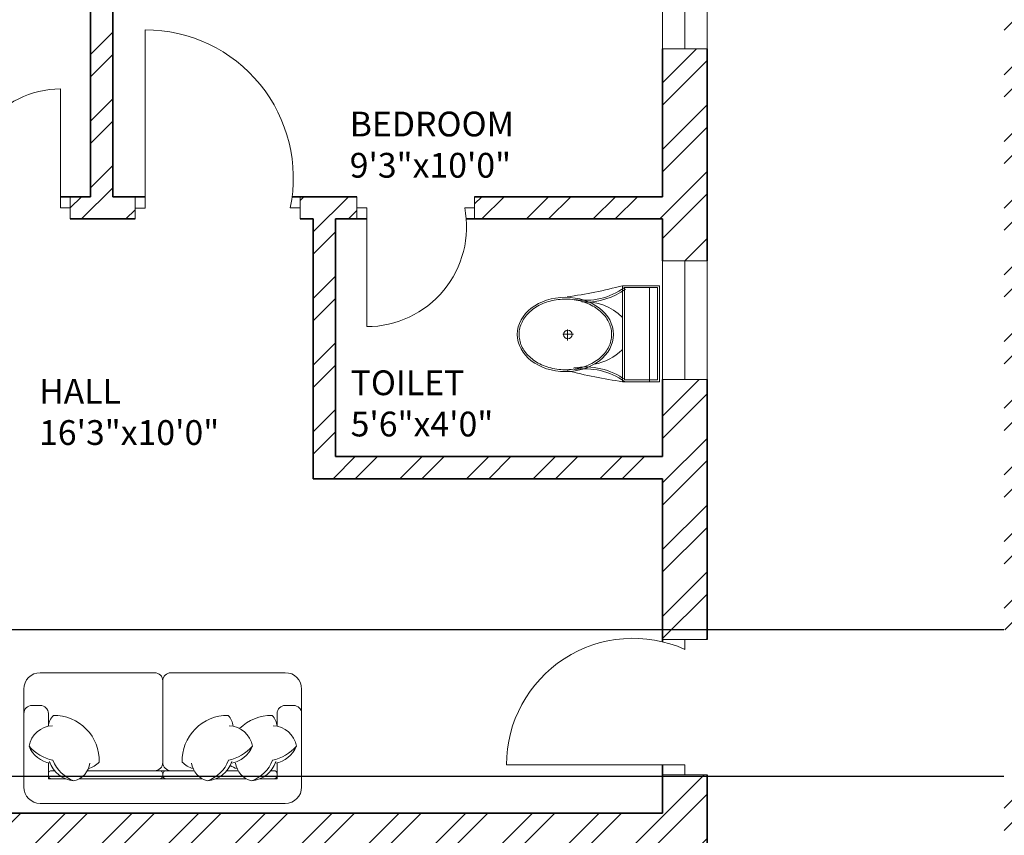
# Model space of a CAD drawing. Units: inches. Extents: x 2552 to 3217, y 1417 to 2737.
# Tile 18 of 25: x 2710 to 2909, y 2392 to 2556. Entities that reach past the tile are written whole.
import ezdxf

# ---------------------------------------------------------------- set-up
doc = ezdxf.new("R2010")
doc.units = ezdxf.units.IN
for name, color, linetype, lineweight in [('A-ANNO-DIMS', 2, 'Continuous', 18), ('A-AREA-IDEN', 7, 'Continuous', 18), ('A-DOOR', 21, 'Continuous', 18), ('A-FLOR-FIXT', 8, 'Continuous', 18), ('A-FURN', 8, 'Continuous', 13), ('A-GLAZ', 161, 'Continuous', 18), ('A-WALL', 7, 'Continuous', 35), ('A-WALL-PATT', 217, 'Continuous', 13)]:
    doc.layers.add(name, color=color, linetype=linetype, lineweight=lineweight)
doc.styles.get("Standard").update_dxf_attribs({"font": 'arial.ttf'})
doc.dimstyles.get("Standard").update_dxf_attribs({"dimtxt": 0.18, "dimasz": 0.18, "dimexe": 0.18, "dimexo": 0.0625, "dimgap": 0.09, "dimtad": 0, "dimtih": 1, "dimtoh": 1, "dimdec": 4, "dimzin": 0, "dimdsep": 46, "dimtxsty": 'Standard', "dimcen": 0.09, "dimadec": 0, "dimazin": 0, "dimtfac": 1, "dimtdec": 4, "dimtofl": 0, "dimtmove": 0, "dimatfit": 3, "dimfxl": 1, "dimtolj": 1, "dimtzin": 0, "dimarcsym": 0})

# ---------------------------------------------------------------- blocks, each defined once
blk = doc.blocks.new('A$C31115884')
for p, q in [((283.1, 497.7), (223.4, 497.7)), ((257.5, 466.4), (257.5, 523.2)), ((0, 200), (0, 0)), ((520, 200), (0, 200)), ((10, 190), (10, 10)), ((510, 190), (10, 190)), ((510, 10), (510, 190)), ((520, 0), (520, 200)), ((510, 54.5), (0, 54.5)), ((10, 10), (510, 10)), ((0, 0), (520, 0))]:
    blk.add_line(p, q)
blk.add_circle((255.6, 496.4), 23.6)
for centre, radius, start, end in [((2777.7, -204.6), 2807, 165.4549, 171.7133), ((3237, 905), 2807, 188.2867, 194.5451), ((-294.5, 403.3), 364.7, 324.2091, 9.3499), ((-294.5, 403.3), 374.7, 324.2091, 9.3499), ((805.8, 403.3), 364.7, 170.6501, 215.7909), ((139.5, 406.2), 293.5, 315.8436, 2.6563), ((805.8, 403.3), 374.7, 179.2036, 215.7909), ((383.6, 406.2), 293.5, 190.2774, 224.1564)]:
    blk.add_arc(centre, radius, start, end)
blk.add_ellipse((256.2, 509.9), major_axis=(0, -260.7), ratio=0.772727)
blk.add_open_spline([(256.2, 259.2), (263.1, 259.2), (270, 259.7), (287.8, 262.3), (298.7, 265.1), (319.9, 273.1), (330.2, 278.4), (350.1, 291.1), (359.7, 298.7), (377.7, 315.9), (386.2, 325.5), (401.7, 346.6), (408.8, 358.1), (421.3, 382.5), (426.8, 395.5), (435.9, 422.4), (439.5, 436.4), (444.8, 465.1), (446.5, 479.7), (447.9, 509.2), (447.6, 524), (445, 553.3), (442.7, 567.8), (436.3, 596), (432.1, 609.7), (421.9, 636), (416, 648.6), (402.5, 672.1), (395, 683), (378.6, 703), (369.8, 712.1), (351.1, 728), (341.3, 734.8), (320.9, 746.2), (310.4, 750.7), (288.9, 757.3), (278, 759.4), (256, 761), (245, 760.6), (223.1, 757.2), (212.3, 754.3), (191.1, 746.1), (180.8, 740.7), (160.9, 727.8), (151.4, 720.1), (133.5, 702.7), (125.1, 693), (109.6, 671.7), (102.6, 660.2), (90.2, 635.7), (84.9, 622.7), (76, 595.6), (72.4, 581.6), (67.2, 552.9), (65.6, 538.2), (64.4, 508.8), (64.8, 494), (67.5, 464.7), (69.9, 450.2), (76.6, 422), (80.8, 408.3), (91.1, 382.2), (97.2, 369.7), (110.8, 346.3), (118.4, 335.4), (134.8, 315.6), (143.7, 306.7), (162.4, 290.9), (172.3, 284.2), (192.8, 273), (203.3, 268.6), (224.8, 262.2), (235.8, 260.2), (249.9, 259.3), (253, 259.2), (256.2, 259.2)], degree=3, knots=[0, 0, 0, 0, 0.110105, 0.110105, 0.285049, 0.285049, 0.459994, 0.459994, 0.634938, 0.634938, 0.809882, 0.809882, 0.984827, 0.984827, 1.159771, 1.159771, 1.334715, 1.334715, 1.50966, 1.50966, 1.684604, 1.684604, 1.859549, 1.859549, 2.034493, 2.034493, 2.209437, 2.209437, 2.384382, 2.384382, 2.559326, 2.559326, 2.73427, 2.73427, 2.909215, 2.909215, 3.084159, 3.084159, 3.259103, 3.259103, 3.434048, 3.434048, 3.608992, 3.608992, 3.783936, 3.783936, 3.958881, 3.958881, 4.133825, 4.133825, 4.30877, 4.30877, 4.483714, 4.483714, 4.658658, 4.658658, 4.833603, 4.833603, 5.008547, 5.008547, 5.183491, 5.183491, 5.358436, 5.358436, 5.53338, 5.53338, 5.708324, 5.708324, 5.883269, 5.883269, 6.058213, 6.058213, 6.233158, 6.233158, 6.283185, 6.283185, 6.283185, 6.283185])
blk = doc.blocks.new('WIN-24')
for p, q in [((0, 24), (9, 24)), ((0, 24), (0, 0)), ((9, 24), (4.5, 24)), ((4.5, 24), (4.5, 0)), ((9, 24), (9, 0)), ((4.5, 0), (0, 0)), ((0, 0), (9, 0))]:
    blk.add_line(p, q)
blk = doc.blocks.new('WIN-48-ALT')
for p, q in [((0, 0), (0, 9)), ((0, 9), (0, 4.5)), ((0, 9), (48, 9)), ((48, 4.5), (48, 9)), ((48, 9), (48, 0)), ((0, 4.5), (48, 4.5)), ((0, 0), (48, 0))]:
    blk.add_line(p, q)
blk = doc.blocks.new('*D55')
at = {"layer": 'A-ANNO-DIMS', "color": 0, "lineweight": -2, "transparency": 16777216}
for p, q in [((2908.79, 2433), (2577.37, 2433)), ((2577.55, 2432.82), (2577.55, 2418.39)), ((2577.55, 2403.59), (2577.55, 2418.02)), ((2908.79, 2403.41), (2577.37, 2403.41))]:
    blk.add_line(p, q, dxfattribs=at)
at = {"layer": 'A-ANNO-DIMS', "color": 0, "transparency": 16777216}
for points in [[(2577.52, 2432.82), (2577.58, 2432.82), (2577.55, 2433)], [(2577.52, 2403.59), (2577.58, 2403.59), (2577.55, 2403.41)]]:
    blk.add_solid(points, dxfattribs=at)
at = {"layer": 'Defpoints', "color": 0, "transparency": 16777216}
for p in [(2577.55, 2433), (2908.85, 2433), (2908.85, 2403.41)]:
    blk.add_point(p, dxfattribs=at)
at = {"layer": 'A-ANNO-DIMS', "color": 0, "transparency": 16777216, "insert": (2577.55, 2418.21), "char_height": 0.18, "attachment_point": 5}
blk.add_mtext('\\A1;29.59', dxfattribs=at)
blk = doc.blocks.new('*D64')
at = {"layer": 'A-ANNO-DIMS', "color": 0, "lineweight": -2, "transparency": 16777216}
for p, q in [((2646.35, 1551.58), (2646.35, 2709.49)), ((2646.53, 2709.31), (2802.77, 2709.31)), ((2959.93, 2709.31), (2803.69, 2709.31)), ((2960.11, 1551.58), (2960.11, 2709.49))]:
    blk.add_line(p, q, dxfattribs=at)
at = {"layer": 'A-ANNO-DIMS', "color": 0, "transparency": 16777216}
for points in [[(2646.53, 2709.34), (2646.53, 2709.28), (2646.35, 2709.31)], [(2959.93, 2709.34), (2959.93, 2709.28), (2960.11, 2709.31)]]:
    blk.add_solid(points, dxfattribs=at)
at = {"layer": 'Defpoints', "color": 0, "transparency": 16777216}
for p in [(2960.11, 2709.31), (2646.35, 1551.51), (2960.11, 1551.51)]:
    blk.add_point(p, dxfattribs=at)
at = {"layer": 'A-ANNO-DIMS', "color": 0, "transparency": 16777216, "insert": (2803.23, 2709.31), "char_height": 0.18, "attachment_point": 5}
blk.add_mtext('\\A1;313.76', dxfattribs=at)
blk = doc.blocks.new('*D69')
at = {"layer": 'A-ANNO-DIMS', "color": 0, "lineweight": -2, "transparency": 16777216}
for p, q in [((2908.79, 2403.41), (2577.37, 2403.41)), ((2577.55, 2403.23), (2577.55, 2395.39)), ((2577.55, 2387.19), (2577.55, 2395.03)), ((2917.79, 2387.01), (2577.37, 2387.01))]:
    blk.add_line(p, q, dxfattribs=at)
at = {"layer": 'A-ANNO-DIMS', "color": 0, "transparency": 16777216}
for points in [[(2577.52, 2403.23), (2577.58, 2403.23), (2577.55, 2403.41)], [(2577.52, 2387.19), (2577.58, 2387.19), (2577.55, 2387.01)]]:
    blk.add_solid(points, dxfattribs=at)
at = {"layer": 'Defpoints', "color": 0, "transparency": 16777216}
for p in [(2577.55, 2403.41), (2908.85, 2403.41), (2917.85, 2387.01)]:
    blk.add_point(p, dxfattribs=at)
at = {"layer": 'A-ANNO-DIMS', "color": 0, "transparency": 16777216, "insert": (2577.55, 2395.21), "char_height": 0.18, "attachment_point": 5}
blk.add_mtext('\\A1;16.4', dxfattribs=at)

msp = doc.modelspace()

# ---------------------------------------------------------------- hatches: boundary and pattern name
at = {"layer": 'A-WALL-PATT'}
h = msp.add_hatch(dxfattribs=at)
h.set_pattern_fill('ANSI32', color=256)
h.paths.add_polyline_path([(2756.676, 2649.5125), (2637.3535, 2649.5125), (2637.3535, 2617.9626), (2641.8535, 2617.9626), (2646.3535, 2617.9626), (2646.3535, 2640.5125), (2724.3535, 2640.5125), (2724.3535, 2520.5125), (2720.299, 2520.5125), (2720.299, 2516.0125), (2733.4075, 2516.0125), (2733.4075, 2518.2213), (2733.4075, 2520.5125), (2728.8535, 2520.5125), (2728.8535, 2640.5125), (2756.676, 2640.5125)])
h.paths.add_polyline_path([(2848.8535, 2649.5125), (2804.676, 2649.5125), (2804.676, 2640.5125), (2839.8535, 2640.5125), (2839.8535, 2598.3517), (2848.8535, 2598.3517)])
h.paths.add_polyline_path([(2646.3535, 2516.0125), (2697.9593, 2516.0125), (2697.9593, 2518.2625), (2697.9593, 2520.5125), (2646.3535, 2520.5125), (2646.3535, 2581.9626), (2637.3535, 2581.9626), (2637.3535, 2364.3298), (2646.3535, 2364.3298), (2646.3535, 2387.0125), (2724.3535, 2387.0125), (2724.3535, 2267.0125), (2721.0443, 2267.0125), (2721.0443, 2262.5125), (2733.7854, 2262.5125), (2733.7854, 2264.7625), (2733.7854, 2267.0125), (2728.8535, 2267.0125), (2728.8535, 2387.0125), (2839.8535, 2387.0125), (2839.8535, 2363.8387), (2848.8535, 2363.8387), (2848.8535, 2403.7415), (2844.3535, 2403.7415), (2839.8535, 2403.7415), (2839.8535, 2396.0125), (2646.3535, 2396.0125)])
h.paths.add_polyline_path([(2848.8535, 2550.3517), (2844.3535, 2550.3517), (2839.8535, 2550.3517), (2839.8535, 2520.5125), (2801.9195, 2520.5125), (2801.9195, 2518.2625), (2801.9195, 2516.0125), (2839.8535, 2516.0125), (2839.8535, 2507.5813), (2848.8535, 2507.5813)], flags=17)
h.paths.add_polyline_path([(2848.8535, 2483.5813), (2844.3535, 2483.5813), (2839.8535, 2483.5813), (2839.8535, 2468.0125), (2773.8535, 2468.0125), (2773.8535, 2516.0125), (2778.1336, 2516.0125), (2778.1336, 2520.5125), (2766.696, 2520.5125), (2766.696, 2518.2625), (2766.696, 2516.0125), (2769.3535, 2516.0125), (2769.3535, 2463.5125), (2839.8535, 2463.5125), (2839.8535, 2431.0782), (2848.8535, 2431.0782)], flags=17)
h.paths.add_polyline_path([(2917.8535, 2569.2764), (2913.3535, 2569.2764), (2908.8535, 2569.2764), (2908.8535, 2433.001), (2917.8535, 2433.001), (2917.8535, 2516.0125), (2967.486, 2516.0125), (2967.486, 2520.5125), (2917.8535, 2520.5125)])
h.paths.add_polyline_path([(3000.3535, 2640.5125), (2995.8535, 2640.5125), (2995.8535, 2520.5125), (2990.688, 2520.5125), (2990.688, 2516.0125), (3004.0844, 2516.0125), (3004.0844, 2518.2625), (3004.0844, 2520.5125), (3000.3535, 2520.5125)])
h.paths.add_polyline_path([(3120.3535, 2561.3689), (3115.8535, 2561.3689), (3111.3535, 2561.3689), (3111.3535, 2520.5125), (3070.9814, 2520.5125), (3070.9814, 2518.2625), (3070.9814, 2516.0125), (3111.3535, 2516.0125), (3111.3535, 2505.1841), (3120.3535, 2505.1841)])
h.paths.add_polyline_path([(3120.3535, 2481.1841), (3115.8535, 2481.1841), (3111.3535, 2481.1841), (3111.3535, 2468.0125), (3045.3535, 2468.0125), (3045.3535, 2516.0125), (3048.9787, 2516.0125), (3048.9787, 2520.5125), (3036.3395, 2520.5125), (3036.3395, 2516.0125), (3040.8535, 2516.0125), (3040.8535, 2463.5125), (3111.3535, 2463.5125), (3111.3535, 2396.0125), (2917.8535, 2396.0125), (2917.8535, 2403.4124), (2913.3535, 2403.4124), (2908.8535, 2403.4124), (2908.8535, 2182.5756), (2917.8535, 2182.5756), (2917.8535, 2262.5125), (2968.001, 2262.5125), (2968.001, 2264.7625), (2968.001, 2267.0125), (2917.8535, 2267.0125), (2917.8535, 2387.0125), (3111.3535, 2387.0125), (3111.3535, 2352.2435), (3120.3535, 2352.2435)])
h.paths.add_polyline_path([(3120.3535, 2304.2435), (3115.8535, 2304.2435), (3111.3535, 2304.2435), (3111.3535, 2267.0125), (3073.8616, 2267.0125), (3073.8616, 2264.7625), (3073.8616, 2262.5125), (3111.3535, 2262.5125), (3111.3535, 2252.376), (3120.3535, 2252.376)], flags=17)
h.paths.add_polyline_path([(3120.3535, 2228.376), (3115.8535, 2228.376), (3111.3535, 2228.376), (3111.3535, 2214.5125), (3045.3535, 2214.5125), (3045.3535, 2262.5125), (3049.3096, 2262.5125), (3049.3096, 2267.0125), (3035.0125, 2267.0125), (3035.0125, 2262.5125), (3040.8535, 2262.5125), (3040.8535, 2210.0125), (3111.3535, 2210.0125), (3111.3535, 2142.5125), (2917.8535, 2142.5125), (2917.8535, 2150.2408), (2913.3535, 2150.2408), (2908.8535, 2150.2408), (2908.8535, 1924.9905), (2917.8535, 1924.9905), (2917.8535, 2009.0125), (2971.959, 2009.0125), (2971.959, 2011.2625), (2971.959, 2013.5125), (2917.8535, 2013.5125), (2917.8535, 2133.5125), (2995.8535, 2133.5125), (2995.8535, 2013.5125), (2992.1797, 2013.5125), (2992.1797, 2009.0125), (3004.3344, 2009.0125), (3004.3344, 2011.2625), (3004.3344, 2013.5125), (3000.3535, 2013.5125), (3000.3535, 2133.5125), (3111.3535, 2133.5125), (3111.3535, 2115.0291), (3120.3535, 2115.0291)])
h.paths.add_polyline_path([(3000.3535, 2387.0125), (2995.8535, 2387.0125), (2995.8535, 2267.0125), (2991.3326, 2267.0125), (2991.3326, 2262.5125), (3004.1044, 2262.5125), (3004.1044, 2264.7625), (3004.1044, 2267.0125), (3000.3535, 2267.0125)], flags=17)
h.paths.add_polyline_path([(3120.3535, 1973.2388), (3115.8535, 1973.2388), (3111.3535, 1973.2388), (3111.3535, 1961.0125), (3045.3535, 1961.0125), (3045.3535, 2009.0125), (3048.9101, 2009.0125), (3048.9101, 2013.5125), (3037.105, 2013.5125), (3037.105, 2011.2625), (3037.105, 2009.0125), (3040.8535, 2009.0125), (3040.8535, 1956.5125), (3111.3535, 1956.5125), (3111.3535, 1889.0125), (2917.8535, 1889.0125), (2917.8535, 1895.7215), (2913.3535, 1895.7215), (2908.8535, 1895.7215), (2908.8535, 1844.2217), (2917.8535, 1844.2217), (2917.8535, 1880.0125), (3111.3535, 1880.0125), (3111.3535, 1846.9541), (3120.3535, 1846.9541)])
h.paths.add_polyline_path([(3120.3535, 2067.0291), (3111.3535, 2067.0291), (3111.3535, 2013.5125), (3071.3001, 2013.5125), (3071.3001, 2009.0125), (3111.3535, 2009.0125), (3111.3535, 1997.2388), (3120.3535, 1997.2388)], flags=0)
h.paths.add_polyline_path([(3120.3535, 1798.9541), (3115.8535, 1798.9541), (3111.3535, 1798.9541), (3111.3535, 1760.0125), (3071.2497, 1760.0125), (3071.2497, 1757.7625), (3071.2497, 1755.5125), (3111.3535, 1755.5125), (3111.3535, 1746.162), (3120.3535, 1746.2478)])
h.paths.add_polyline_path([(3120.3535, 1722.2049), (3111.3535, 1722.2049), (3111.3535, 1707.5125), (3045.3535, 1707.5125), (3045.3535, 1755.5125), (3048.6624, 1755.5125), (3048.6624, 1760.0125), (3035.3703, 1760.0125), (3035.3703, 1755.5125), (3040.8535, 1755.5125), (3040.8535, 1703.0125), (3111.3535, 1703.0125), (3111.3535, 1635.5125), (2917.8535, 1635.5125), (2917.8535, 1643.1366), (2913.3535, 1643.1366), (2908.8535, 1643.1366), (2908.8535, 1626.5125), (3120.3535, 1626.5125)])
h.paths.add_polyline_path([(2917.8535, 1755.5125), (2973.2287, 1755.5125), (2973.2287, 1757.7625), (2973.2287, 1760.0125), (2917.8535, 1760.0125), (2917.8535, 1808.2217), (2913.3535, 1808.2217), (2908.8535, 1808.2217), (2908.8535, 1676.1665), (2917.8535, 1676.1665)])
h.paths.add_polyline_path([(3000.3535, 1880.0125), (2995.8535, 1880.0125), (2995.8535, 1760.0125), (2992.9329, 1760.0125), (2992.9329, 1755.5125), (3003.8766, 1755.5125), (3003.8766, 1757.7625), (3003.8766, 1760.0125), (3000.3535, 1760.0125)])
h.paths.add_polyline_path([(2848.8535, 1896.6971), (2844.3535, 1896.6971), (2839.8535, 1896.6971), (2839.8535, 1889.0125), (2646.3535, 1889.0125), (2646.3535, 2009.0125), (2700.5253, 2009.0125), (2700.5253, 2011.2625), (2700.5253, 2013.5125), (2646.3535, 2013.5125), (2646.3535, 2053.1812), (2641.8535, 2053.1812), (2637.3535, 2053.1812), (2637.3535, 1836.254), (2646.3535, 1836.254), (2646.3535, 1880.0125), (2724.3535, 1880.0125), (2724.3535, 1760.0125), (2721.2473, 1760.0125), (2721.2473, 1755.5125), (2731.9187, 1755.5125), (2731.9187, 1757.7625), (2731.9187, 1760.0125), (2728.8535, 1760.0125), (2728.8535, 1880.0125), (2839.8535, 1880.0125), (2839.8535, 1840.3813), (2848.8535, 1840.3813)])
h.paths.add_polyline_path([(2848.8535, 1792.3813), (2844.3535, 1792.3813), (2839.8535, 1792.3813), (2839.8535, 1760.0125), (2797.8845, 1760.0125), (2797.8845, 1755.5125), (2839.8535, 1755.5125), (2839.8535, 1743.3688), (2844.3535, 1743.3688), (2848.8535, 1743.3688)], flags=0)
h.paths.add_polyline_path([(2848.8535, 1719.3688), (2844.3535, 1719.3688), (2839.8535, 1719.3688), (2839.8535, 1707.5125), (2773.8535, 1707.5125), (2773.8535, 1755.5125), (2777.716, 1755.5125), (2777.716, 1760.0125), (2760.9247, 1760.0125), (2760.9247, 1757.9721), (2760.9247, 1755.5125), (2769.3535, 1755.5125), (2769.3535, 1703.0125), (2839.8535, 1703.0125), (2839.8535, 1673.0277), (2848.8535, 1672.9407)], flags=0)
h.paths.add_polyline_path([(2646.3535, 1755.5125), (2702.9171, 1755.5125), (2702.9171, 1757.7625), (2702.9171, 1760.0125), (2646.3535, 1760.0125), (2646.3535, 1800.254), (2641.8535, 1800.254), (2637.3535, 1800.254), (2637.3535, 1626.5125), (2848.8535, 1626.5125), (2848.8535, 1643.1187), (2844.3535, 1643.1187), (2839.8535, 1643.1187), (2839.8535, 1635.5125), (2646.3535, 1635.5125)])
h.paths.add_polyline_path([(2848.8535, 2148.8427), (2844.3535, 2148.8427), (2839.8535, 2148.8427), (2839.8535, 2142.5125), (2646.3535, 2142.5125), (2646.3535, 2262.5125), (2701.3562, 2262.5125), (2701.3562, 2264.7625), (2701.3562, 2267.0125), (2646.3535, 2267.0125), (2646.3535, 2328.3298), (2637.3535, 2328.3298), (2637.3535, 2089.1812), (2646.3535, 2089.1812), (2646.3535, 2133.5125), (2839.8535, 2133.5125), (2839.8535, 2097.5966), (2848.8535, 2097.5966)])
h.paths.add_polyline_path([(2728.8535, 2133.5125), (2724.3535, 2133.5125), (2724.3535, 2013.5125), (2719.6039, 2013.5125), (2719.6039, 2009.0125), (2732.5784, 2009.0125), (2732.5784, 2011.2625), (2732.5784, 2013.5125), (2728.8535, 2013.5125)])
h.paths.add_polyline_path([(2848.8535, 1970.0557), (2844.3535, 1970.0557), (2839.8535, 1970.0557), (2839.8535, 1961.0125), (2773.8535, 1961.0125), (2773.8535, 2009.0125), (2777.3388, 2009.0125), (2777.3388, 2013.5125), (2764.7681, 2013.5125), (2764.7681, 2009.0125), (2769.3535, 2009.0125), (2769.3535, 1956.5125), (2839.8535, 1956.5125), (2839.8535, 1924.7199), (2848.8535, 1924.7199)], flags=17)
h.paths.add_polyline_path([(2848.8535, 2049.5966), (2844.3535, 2049.5966), (2839.8535, 2049.5966), (2839.8535, 2013.5125), (2798.198, 2013.5125), (2798.198, 2011.2625), (2798.198, 2009.0125), (2839.8535, 2009.0125), (2839.8535, 1994.0557), (2848.8535, 1994.0557)], flags=17)
h.paths.add_polyline_path([(2848.8535, 2315.8387), (2839.8535, 2315.8387), (2839.8535, 2267.0125), (2799.3375, 2267.0125), (2799.3375, 2264.7625), (2799.3375, 2262.5125), (2839.8535, 2262.5125), (2839.8535, 2253.2843), (2848.8535, 2253.2843)], flags=17)
h.paths.add_polyline_path([(2848.8535, 2229.2843), (2839.8535, 2229.2843), (2839.8535, 2177.6936), (2848.8535, 2177.6936)], flags=17)
h.paths.add_polyline_path([(2839.8535, 2214.5125), (2773.8535, 2214.5125), (2773.8535, 2262.5125), (2777.6984, 2262.5125), (2777.6984, 2267.0125), (2763.8226, 2267.0125), (2763.8226, 2262.5125), (2769.3535, 2262.5125), (2769.3535, 2210.0125), (2839.8535, 2210.0125)], flags=17)
h.paths.add_polyline_path([(3050.32, 2520.2817), (3088.9114, 2520.2817), (3088.9114, 2538.939), (3050.32, 2538.939)], flags=9)

# ---------------------------------------------------------------- linework, layer by layer
at = {"layer": 'A-DOOR'}
for p, q in [((2735.4075, 2518.2213), (2735.4075, 2554.2213)), ((2718.299, 2518.2625), (2718.299, 2542.2625)), ((2720.299, 2520.5125), (2720.299, 2516.0125)), ((2733.4075, 2520.5125), (2733.4075, 2516.6327)), ((2766.696, 2516.0125), (2766.696, 2520.5125)), ((2766.696, 2520.5125), (2766.696, 2518.2625)), ((2778.1336, 2516.0125), (2778.1336, 2520.5125)), ((2778.1336, 2520.5125), (2778.1336, 2518.2625)), ((2801.9195, 2516.0125), (2801.9195, 2520.5125)), ((2801.9195, 2520.5125), (2801.9195, 2518.2625)), ((2720.299, 2518.2625), (2718.299, 2518.2625)), ((2720.299, 2516.0125), (2720.299, 2518.2625)), ((2733.4075, 2516.0125), (2733.4075, 2518.2213)), ((2733.4075, 2518.2213), (2735.4075, 2518.2213)), ((2733.4075, 2516.6327), (2733.4075, 2516.0125)), ((2766.696, 2518.2625), (2764.696, 2518.2625)), ((2778.1336, 2518.2625), (2780.1336, 2518.2625)), ((2780.1336, 2518.2625), (2780.1336, 2494.2625)), ((2801.9195, 2518.2625), (2799.9195, 2518.2625)), ((2839.8535, 2431.0782), (2848.8535, 2431.0782)), ((2848.8535, 2431.0782), (2844.3535, 2431.0782)), ((2844.3535, 2431.0782), (2844.3535, 2429.0782)), ((2844.3535, 2405.7415), (2808.3535, 2405.7415)), ((2844.3535, 2403.7415), (2844.3535, 2405.7415)), ((2839.8535, 2403.7415), (2848.8535, 2403.7415)), ((2848.8535, 2403.7415), (2844.3535, 2403.7415))]:
    msp.add_line(p, q, dxfattribs=at)
for centre, radius, start, end in [((2735.4075, 2524.3142), 29.9071, 348.325673, 90), ((2718.299, 2523.2554), 19.0071, 90, 195.22938), ((2780.1336, 2514.4184), 20.1559, 270, 10.994764), ((2833.9174, 2405.7415), 25.5639, 65.906008, 180)]:
    msp.add_arc(centre, radius, start, end, dxfattribs=at)
at = {"layer": 'A-FURN', "ltscale": 0.03}
msp.add_lwpolyline([(2737.3083, 2424.3613, -0.41421356), (2738.9579, 2422.7117, -0.41421356), (2740.6074, 2424.3613), (2763.7013, 2424.3613, -0.41421356), (2767.0005, 2421.0621), (2767.0005, 2401.2674, -0.41421356), (2763.7013, 2397.9683), (2714.2144, 2397.9683, -0.41421356), (2710.9153, 2401.2674), (2710.9153, 2421.0621, -0.41421356), (2714.2144, 2424.3613), (2737.3083, 2424.3613, -0.41421356), (2738.9579, 2422.7117, -0.41421356), (2740.6074, 2424.3613)], format="xyb", dxfattribs=at)
at = {"layer": 'A-FURN'}
for points in [[(2737.3083, 2404.5665, 0.41421356), (2738.9579, 2406.2161), (2738.9579, 2422.7117, 0.41421356)], [(2740.6074, 2404.5665, -0.41421356), (2738.9579, 2406.2161), (2738.9579, 2422.7117, -0.41421356)], [(2710.9153, 2416.1135, -0.41421356), (2712.5649, 2417.763), (2714.2144, 2417.763, -0.41421356), (2715.864, 2416.1135), (2715.864, 2413.5577)], [(2762.0518, 2413.5577), (2762.0518, 2416.1135, -0.41421356), (2763.7013, 2417.763), (2765.3509, 2417.763, -0.41421356), (2767.0005, 2416.1135)], [(2715.8604, 2413.5569, -0.16554063), (2716.8809, 2415.7365, -0.42598917), (2726.1451, 2406.2867, -0.12152332), (2723.946, 2404.9842, 7.11546429)], [(2753.1692, 2413.5569, 0.16554063), (2752.1487, 2415.7365, 0.42598917), (2742.8845, 2406.2867, 0.12152332), (2745.0836, 2404.9842, -7.11546429)], [(2762.0554, 2413.5569, 0.16554063), (2761.0349, 2415.7365, 0.20023115), (2754.4867, 2413.082, 0.12152332)], [(2716.6918, 2413.6575, 0.35677236), (2711.9651, 2409.4996, 0.24954205), (2716.2479, 2406.0731, -9.61688035)], [(2752.3378, 2413.6575, -0.35677236), (2757.0645, 2409.4996, -0.24954205), (2752.7817, 2406.0731, 9.61688035)], [(2761.2239, 2413.6575, -0.35677236), (2765.9506, 2409.4996, -0.24954205), (2761.6678, 2406.0731, 9.61688035)], [(2711.9651, 2409.4996, 0.14772988), (2716.7863, 2406.6647, 0.21334276), (2721.0403, 2402.5067, 0.17866181)], [(2757.0645, 2409.4996, -0.14772988), (2752.2433, 2406.6647, -0.21334276), (2747.9893, 2402.5067, -0.17866181)], [(2765.9506, 2409.4996, -0.14772988), (2761.1294, 2406.6647, -0.21334276), (2756.8754, 2402.5067, -0.17866181)], [(2716.1203, 2406.4387, 0.30666349), (2721.0403, 2402.5067, 0.30632997), (2724.2545, 2406.0977, -0.87284716)], [(2737.3083, 2404.5665, 0.41421356), (2738.9579, 2406.2161)], [(2740.6074, 2404.5665, -0.41421356), (2738.9579, 2406.2161)], [(2752.9093, 2406.4387, -0.30666349), (2747.9893, 2402.5067, -0.30632997), (2744.7751, 2406.0977, 0.87284716)], [(2752.5868, 2405.6291, 0.07186538), (2753.9698, 2404.9842, -7.11546429)], [(2761.7955, 2406.4387, -0.30666349), (2756.8754, 2402.5067, -0.30632997), (2753.6613, 2406.0977, 0.87284716)], [(2758.5815, 2402.9169), (2762.0518, 2402.9169), (2762.0518, 2406.1587, -0.41421356)], [(2717.1228, 2404.5665), (2716.5238, 2404.5665, 0.41421356), (2715.864, 2403.9067), (2715.864, 2403.5768, 0.41421356), (2716.5238, 2402.9169)], [(2722.0785, 2402.9169), (2738.298, 2402.9169, 0.41421356), (2738.9579, 2403.5768), (2738.9579, 2403.9067, 0.41421356), (2738.298, 2404.5665), (2723.7395, 2404.5665, 0.41421356)], [(2746.9511, 2402.9169), (2739.6177, 2402.9169, -0.41421356), (2738.9579, 2403.5768), (2738.9579, 2403.9067, -0.41421356), (2739.6177, 2404.5665), (2745.2901, 2404.5665, -0.41421356)], [(2751.9068, 2404.5665), (2754.1763, 2404.5665, -0.41421356)], [(2760.793, 2404.5665), (2761.3919, 2404.5665, -0.41421356), (2762.0518, 2403.9067), (2762.0518, 2403.5768, -0.41421356), (2761.3919, 2402.9169)], [(2716.5238, 2402.9169), (2719.3342, 2402.9169, 0.41421356)], [(2755.8373, 2402.9169), (2749.6954, 2402.9169, -0.41421356)], [(2761.3919, 2402.9169), (2758.5815, 2402.9169, -0.41421356)]]:
    msp.add_lwpolyline(points, format="xyb", dxfattribs=at)
for points in [[(2715.864, 2406.1587), (2715.864, 2402.9169), (2719.3342, 2402.9169)], [(2722.0785, 2402.9169), (2746.9511, 2402.9169)], [(2749.6954, 2402.9169), (2755.8373, 2402.9169)]]:
    msp.add_lwpolyline(points, dxfattribs=at)
msp.add_lwpolyline([(2738.298, 2402.9169), (2739.6177, 2402.9169, -0.41421356), (2738.9579, 2403.5768), (2738.9579, 2403.9067, -0.41421356), (2739.6177, 2404.5665), (2738.298, 2404.5665, -0.41421356), (2738.9579, 2403.9067), (2738.9579, 2403.5768, -0.41421356)], format="xyb", close=True, dxfattribs=at)
at = {"layer": 'A-WALL'}
for p, q in [((2724.3535, 2640.5125), (2724.3535, 2520.5125)), ((2728.8535, 2640.5125), (2728.8535, 2520.5125)), ((2839.8535, 2550.3517), (2839.8535, 2520.5125)), ((2848.8535, 2550.3517), (2848.8535, 2507.5813)), ((2718.299, 2520.5125), (2724.3535, 2520.5125)), ((2728.8535, 2520.5125), (2735.4075, 2520.5125)), ((2765.072, 2520.5125), (2778.1336, 2520.5125)), ((2801.9195, 2520.5125), (2839.8535, 2520.5125)), ((2720.299, 2516.0125), (2733.4075, 2516.0125)), ((2766.696, 2516.0125), (2769.3535, 2516.0125)), ((2769.3535, 2516.0125), (2769.3535, 2463.5125)), ((2773.8535, 2516.0125), (2773.8535, 2468.0125)), ((2773.8535, 2516.0125), (2780.1336, 2516.0125)), ((2800.2264, 2516.0125), (2839.8535, 2516.0125)), ((2839.8535, 2516.0125), (2839.8535, 2507.5813)), ((2839.8535, 2483.5813), (2839.8535, 2468.0125)), ((2848.8535, 2483.5813), (2848.8535, 2431.0782)), ((2773.8535, 2468.0125), (2839.8535, 2468.0125)), ((2769.3535, 2463.5125), (2839.8535, 2463.5125)), ((2839.8535, 2463.5125), (2839.8535, 2430.6067)), ((2839.8535, 2405.7415), (2839.8535, 2396.0125)), ((2848.8535, 2403.7415), (2848.8535, 2363.8387)), ((2646.3535, 2396.0125), (2839.8535, 2396.0125))]:
    msp.add_line(p, q, dxfattribs=at)

# ---------------------------------------------------------------- block references
at = {"layer": 'A-FLOR-FIXT', "xscale": 0.0372717239612423, "yscale": 0.0372717239612423, "zscale": 0.0372717239612423, "rotation": 89.99999999999999}
msp.add_blockref('A$C31115884', (2839.2439, 2483.1352), dxfattribs=at)
msp.add_blockref('A$C31115884', (2839.2439, 2483.1352), dxfattribs=at)
at = {"layer": 'A-GLAZ', "extrusion": (0, 0, -1), "zscale": -1}
for name, p, rotation in [('WIN-48-ALT', (-2839.854, 2550.3518), 90), ('WIN-24', (-2839.854, 2507.5816), 180)]:
    msp.add_blockref(name, p, dxfattribs=dict(at, rotation=rotation))

# ---------------------------------------------------------------- texts
at = {"layer": 'A-AREA-IDEN', "char_height": 5, "attachment_point": 1}
for s, width, insert in [('BEDROOM\\P9\'3"x10\'0"', 122.578881, (2776.701, 2537.6883)), ('TOILET\\P5\'6"x4\'0"', 71.963486, (2776.89, 2485.4186)), ('HALL\\P16\'3"x10\'0"', 121.730501, (2713.9953, 2483.7046))]:
    msp.add_mtext_dynamic_manual_height_columns(s, width=width, gutter_width=12.5, heights=[0], dxfattribs=dict(at, insert=insert))

# ---------------------------------------------------------------- dimensions: what is measured, and where the dimension line sits
at = {"layer": 'A-ANNO-DIMS'}
dim = msp.add_linear_dim(base=(2960.1089, 2709.3125), p1=(2646.3535, 1551.5125), p2=(2960.1089, 1551.5125), dimstyle='Standard', override={"dimdec": 2, "dimlfac": 1, "dimrnd": 0, "dimzin": 0, "dimdsep": 46, "dimlunit": 2}, dxfattribs=at)
dim.commit()
dim.dimension.update_dxf_attribs({"geometry": '*D64', "text_midpoint": (2803.2312, 2709.3125)})
for base, p1, p2, override, picture, middle in [((2577.5535, 2433.001), (2908.8535, 2403.4124), (2908.8535, 2433.001), {"dimdec": 2, "dimlfac": 1, "dimrnd": 0, "dimzin": 0, "dimdsep": 46, "dimlunit": 2}, '*D55', (2577.5535, 2418.2067)), ((2577.5535, 2403.4124), (2917.8535, 2387.0125), (2908.8535, 2403.4124), {"dimdec": 1, "dimlfac": 1, "dimrnd": 0, "dimzin": 0, "dimdsep": 46, "dimlunit": 2}, '*D69', (2577.5535, 2395.2125))]:
    dim = msp.add_linear_dim(base=base, p1=p1, p2=p2, angle=90, dimstyle='Standard', override=override, dxfattribs=at)
    dim.commit()
    dim.dimension.update_dxf_attribs({"geometry": picture, "text_midpoint": middle})

doc.saveas('drawing.dxf')
